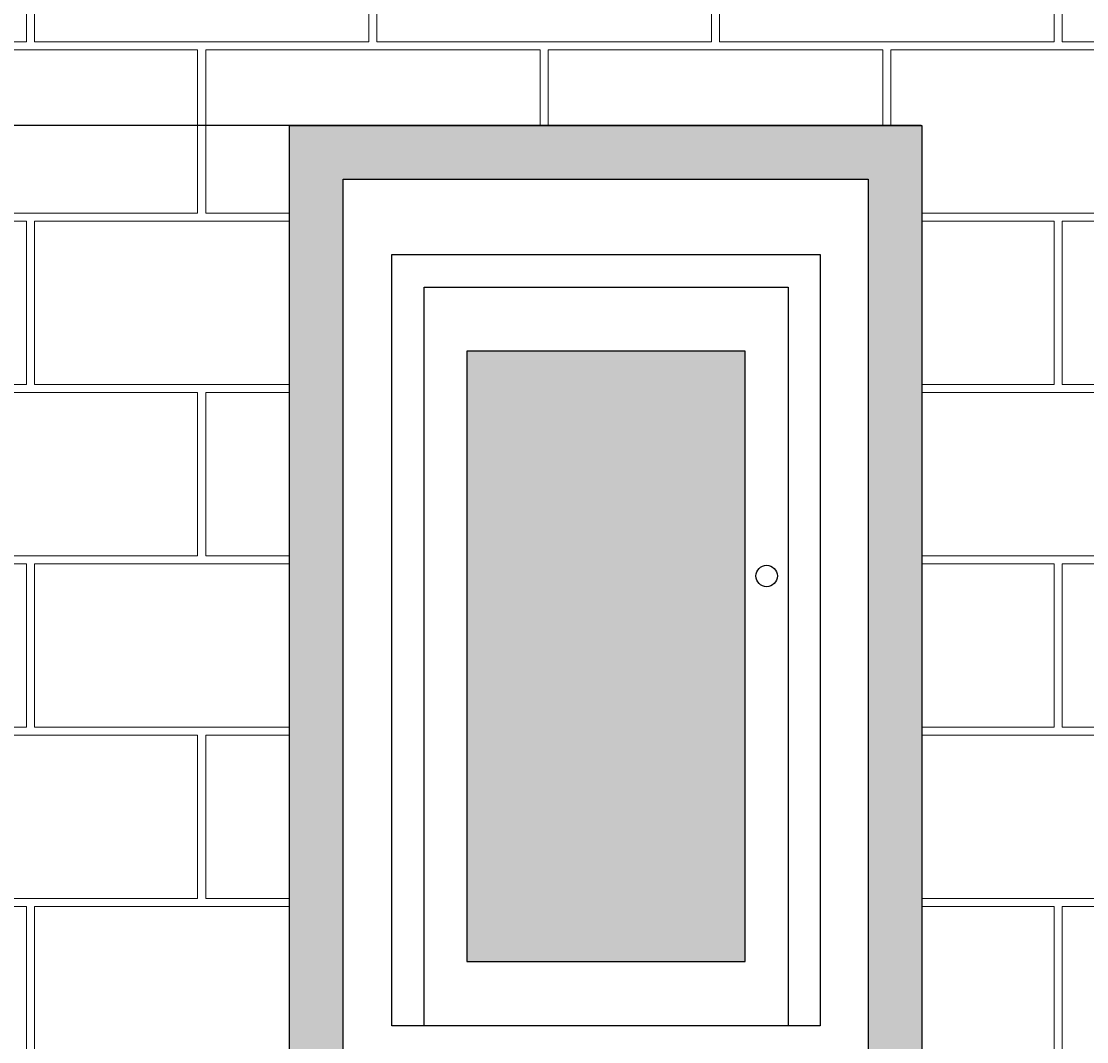
# Model space of a CAD drawing. Units: inches. Extents: x -128 to 854, y -395 to 398.
# Tile 56 of 61: x 467 to 567, y -343 to -248. Entities that reach past the tile are written whole.
import ezdxf

# ---------------------------------------------------------------- set-up
doc = ezdxf.new("R2010")
doc.units = ezdxf.units.IN
doc.header["$MEASUREMENT"] = 0
for name, color, linetype, lineweight in [('A-ANNO-DIMS', 2, 'Continuous', 18), ('A-DOOR', 4, 'Continuous', 25), ('A-ELEV-PATT', 8, 'Continuous', 13)]:
    doc.layers.add(name, color=color, linetype=linetype, lineweight=lineweight)
doc.styles.get("Standard").update_dxf_attribs({"font": 'arial.ttf'})
doc.dimstyles.get("Standard").update_dxf_attribs({"dimtxt": 0.18, "dimasz": 0.18, "dimexe": 0.18, "dimexo": 0.0625, "dimgap": 0.09, "dimtad": 0, "dimtih": 1, "dimtoh": 1, "dimdec": 1, "dimzin": 0, "dimdsep": 46, "dimlunit": 4, "dimtxsty": 'Standard', "dimcen": 0.09, "dimclrd": 1, "dimclre": 2, "dimclrt": 6, "dimadec": 0, "dimazin": 0, "dimtfac": 1, "dimtdec": 1, "dimtofl": 0, "dimtmove": 0, "dimatfit": 3, "dimfxl": 1, "dimtfill": 2, "dimtfillclr": 3, "dimtolj": 1, "dimtzin": 0, "dimarcsym": 0})

# ---------------------------------------------------------------- blocks, each defined once
blk = doc.blocks.new('*U59')
blk.add_lwpolyline([(3.124, 0.013), (0.124, 0.013), (0.124, 72.013), (40.124, 72.013), (40.124, 0.013), (37.124, 0.013)])
for points in [[(37.124, 68.99), (37.124, 0.013), (3.124, 0.013), (3.124, 68.99)], [(33.124, 6.013), (33.124, 62.99), (7.124, 62.99), (7.124, 6.013)]]:
    blk.add_lwpolyline(points, close=True)
blk.add_circle((35.124, 42.013), 1)
blk = doc.blocks.new('*D140')
at = {"layer": 'A-ANNO-DIMS', "color": 2, "lineweight": -2, "transparency": 16777216}
for p, q in [((551.245, -257.476), (346.3, -257.476)), ((551.245, -353.476), (346.3, -353.476))]:
    blk.add_line(p, q, dxfattribs=at)
at = {"layer": 'A-ANNO-DIMS', "color": 1, "lineweight": -2, "transparency": 16777216}
for p, q in [((346.48, -257.656), (346.48, -305.295)), ((346.48, -353.296), (346.48, -305.658))]:
    blk.add_line(p, q, dxfattribs=at)
at = {"layer": 'A-ANNO-DIMS', "color": 1, "transparency": 16777216}
for points in [[(346.45, -257.656), (346.51, -257.656), (346.48, -257.476)], [(346.45, -353.296), (346.51, -353.296), (346.48, -353.476)]]:
    blk.add_solid(points, dxfattribs=at)
at = {"layer": 'Defpoints', "color": 0, "transparency": 16777216}
for p in [(346.48, -257.476), (551.307, -257.476), (551.307, -353.476)]:
    blk.add_point(p, dxfattribs=at)
at = {"layer": 'A-ANNO-DIMS', "color": 6, "transparency": 16777216, "insert": (346.48, -305.476), "char_height": 0.18, "attachment_point": 5, "bg_fill": 1, "box_fill_scale": 1.25, "bg_fill_color": 3, "bg_fill_transparency": 0}
blk.add_mtext('\\A1;8\'-0"', dxfattribs=at)

msp = doc.modelspace()

# ---------------------------------------------------------------- hatches: boundary and pattern name
at = {"layer": 'A-ELEV-PATT'}
h = msp.add_hatch(color=256, dxfattribs=at)
h.dxf.hatch_style = 1
h.paths.add_polyline_path([(418.28, -227.476), (418.28, -233.476), (782.28, -233.476), (782.28, -227.476)])
h.paths.add_polyline_path([(492.252, -257.476), (492.252, -353.476), (551.307, -353.476), (551.307, -257.476)])
h.paths.add_polyline_path([(546.307, -262.476), (546.307, -348.476), (497.252, -348.476), (497.252, -262.476)], flags=16)
h = msp.add_hatch(dxfattribs=at)
h.set_pattern_fill('AR-B816C', color=256, scale=2)
h.set_pattern_definition([(0, (468.407, -10.41), (16, 16), [31.25, -0.75]), (0, (452.407, -9.66), (16, 16), [31.25, -0.75]), (90, (468.407, -10.41), (-16, 16), [-16.75, 15.25]), (90, (467.657, -10.41), (-16, 16), [-16.75, 15.25])])
h.paths.add_polyline_path([(418.28, -353.476), (492.252, -353.476), (492.252, -257.476), (551.307, -257.476), (551.307, -353.476), (782.28, -353.476), (782.28, -233.476), (418.28, -233.476)])
h.paths.add_polyline_path([(668.28, -257.476), (730.28, -257.476), (730.28, -305.476), (668.28, -305.476)], flags=16)
h.paths.add_polyline_path([(673.28, -300.476), (673.28, -262.476), (725.28, -262.476), (725.28, -300.476)], flags=0)
h = msp.add_hatch(color=256, dxfattribs=at)
h.dxf.hatch_style = 1
h.paths.add_polyline_path([(508.818, -335.525), (534.818, -335.525), (534.818, -278.548), (508.818, -278.548)])

# ---------------------------------------------------------------- linework, layer by layer
at = {"layer": 'A-DOOR'}
for points in [[(492.252, -257.476), (551.307, -257.476), (551.307, -353.476), (492.252, -353.476)], [(497.252, -262.476), (546.307, -262.476), (546.307, -348.476), (497.252, -348.476)]]:
    msp.add_lwpolyline(points, close=True, dxfattribs=at)

# ---------------------------------------------------------------- block references
msp.add_blockref('*U59', (501.695, -341.538), dxfattribs=at)

# ---------------------------------------------------------------- dimensions: what is measured, and where the dimension line sits
at = {"layer": 'A-ANNO-DIMS'}
dim = msp.add_linear_dim(base=(346.48, -257.476), p1=(551.307, -353.476), p2=(551.307, -257.476), angle=90, dimstyle='Standard', override={"dimdec": 1, "dimlfac": 1, "dimrnd": 0, "dimzin": 1, "dimdsep": 46, "dimlunit": 4, "dimfrac": 2}, dxfattribs=at)
dim.commit()
dim.dimension.update_dxf_attribs({"geometry": '*D140', "text_midpoint": (346.48, -305.476)})

doc.saveas('drawing.dxf')
